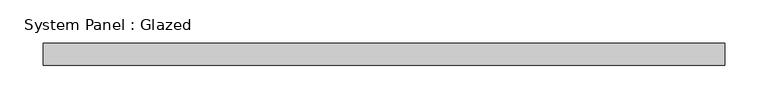
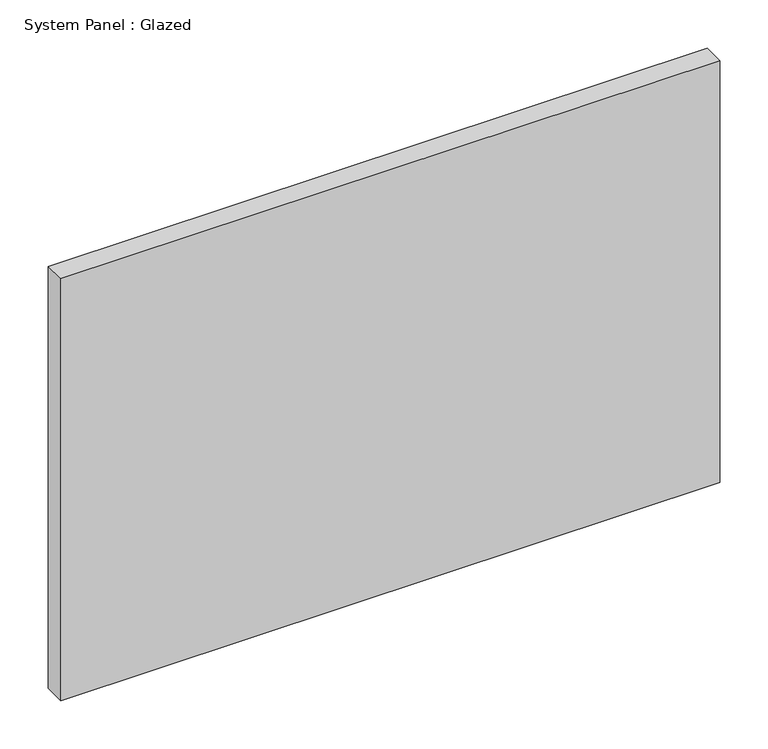
"""IFC4 building model written with IfcOpenShell, lengths in millimetres: plate geometry, System Panel : Glazed."""

from ifc_helpers import new_model, si_unit, origin, origin_with_axes, place, context, project, spatial, polyline, outline, extrude, source, transform, mapped, element, save


def system_panel_glazed_db1fed72(model_context):
    return source(origin(), model_context, "Body", "SweptSolid", [
        extrude(outline(polyline([(393.7, 19.05), (-393.7, 19.05), (-393.7, 44.45), (393.7, 44.45), (393.7, 19.05)])), origin_with_axes(), (0.0, 0.0, 1.0), 533.4059963),
    ])


if __name__ == "__main__":
    model = new_model("IFC4")
    model_context = context("Model", 3, world=origin())
    ifc_project = project(units=[si_unit("LENGTHUNIT", "METRE", prefix="MILLI")], contexts=[model_context])
    site = spatial("IfcSite", under=ifc_project)
    building = spatial("IfcBuilding", under=site)
    placement = place(None, origin())
    system_panel_glazed_shape = system_panel_glazed_db1fed72(model_context)
    element("IfcPlate", 1, ObjectType="System Panel : Glazed", at=placement, inside=building, context=model_context, shape_type="MappedRepresentation", body=[
        mapped(system_panel_glazed_shape, transform((0.0, 0.0, 0.0), x_axis=(1.0, 0.0, 0.0), y_axis=(0.0, 1.0, 0.0), z_axis=(0.0, 0.0, 1.0))),
    ])
    save(model, "model.ifc")

# Revit data of these elements
# Type "System Panel : Glazed"
#   Construction Type Id = "GSP4R"
#   Analytic Construction = "1/8 in Pilkington single glazing"
#   Visual Light Transmittance = 0.9
#   Solar Heat Gain Coefficient = 0.86
#   Heat Transfer Coefficient (U) = 1.18115 BTU/(h·ft²·°F)
#   Define Thermal Properties by = 1
# Element 1 (IfcPlate, "System Panel : Glazed")
#   Materials on its faces: "Glass"
# Materials
#   "Glass": class "Glass", colour RGB 0 128 192, transparency 0.75, Description = "Soda Lime Glass", Cost = 0
